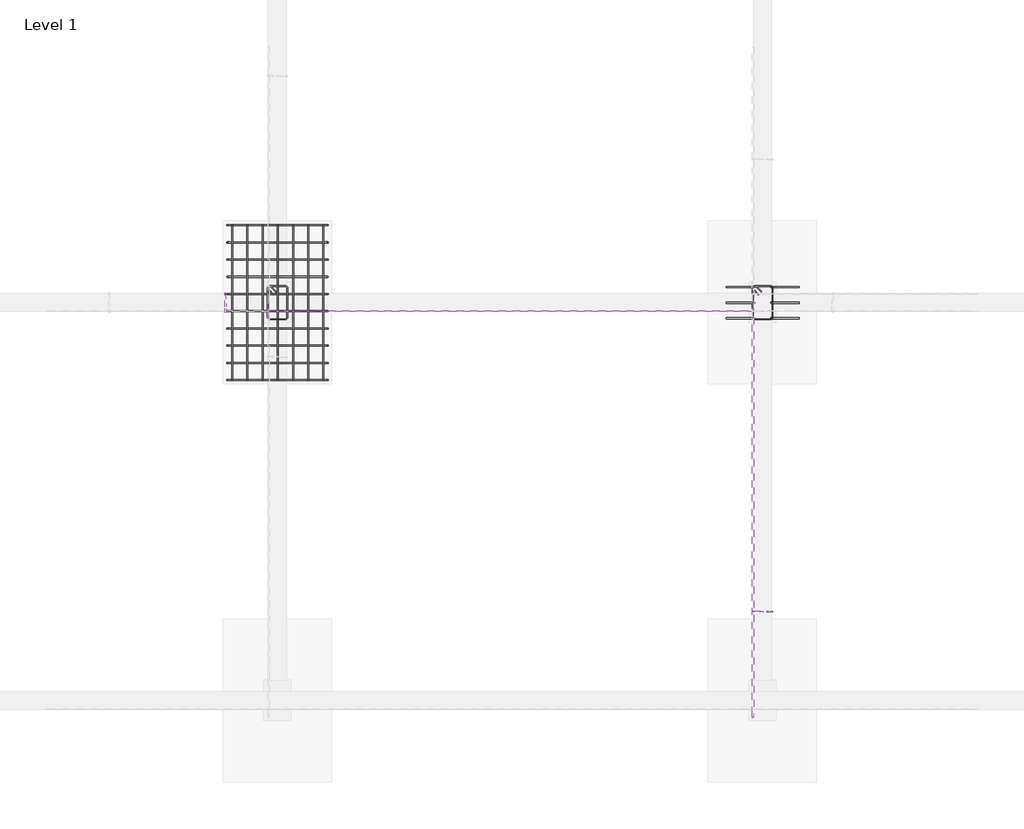
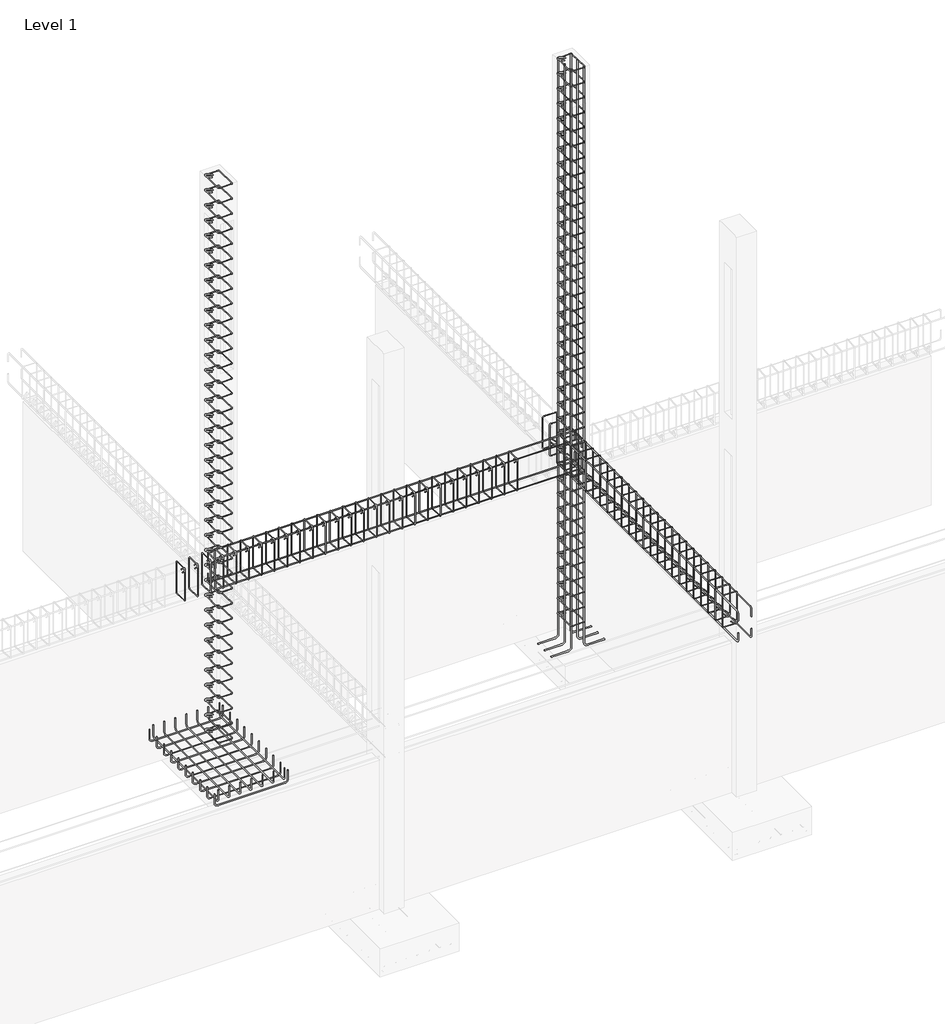
# One storey, part 5 of 8: 12 reinforcing bars.
"""IFC4 building model written with IfcOpenShell, lengths in millimetres."""

from ifc_helpers import new_model, si_unit, point, frame, origin, place, context, project, spatial, polyline, circle_curve, trimmed, segment, composite_curve, source, transform, mapped, element, save
from ifc_brep_helpers import swept_disk

model = new_model("IFC4")

# Units and contexts
model_context = context("Model", 3, world=origin())
ifc_project = project(units=[si_unit("LENGTHUNIT", "METRE", prefix="MILLI")], contexts=[model_context])

# Site, building, storey
site = spatial("IfcSite", under=ifc_project)
building = spatial("IfcBuilding", under=site)
storey = spatial("IfcBuildingStorey", under=building, Name="Level 1", Elevation=0.0)

# Reinforcing bars
placement = place(None, origin())
reinforcing_bar_shape = source(origin(), model_context, "Body", "SolidModel", [
    swept_disk(composite_curve([segment(polyline([(-8817.2482157, 7767.9070829, 9105.9), (-8817.2482157, 7767.9070829, -307.9115)]), True, "CONTINUOUS"), segment(trimmed(circle_curve(frame((-8771.1472157, 7767.9070829, -307.9115), z_axis=(0.0, -1.0, 0.0), x_axis=(-46.10099999999875, 0.0, 0.0)), 46.101), [point((-8817.2482157, 7767.9070829, -307.9115))], [point((-8771.1472157, 7767.9070829, -354.0125))], True, "CARTESIAN"), True, "CONTINUOUS"), segment(polyline([(-8771.1472157, 7767.9070829, -354.0125), (-8504.5742157, 7767.9070829, -354.0125)]), True, "CONTINUOUS")], self_intersect=False), 8.001),
])
element("IfcReinforcingBar", 1, at=placement, inside=storey, context=model_context, shape_type="MappedRepresentation", body=[
    mapped(reinforcing_bar_shape, transform((0.0, 0.0, 0.0), x_axis=(1.0, 0.0, 0.0), y_axis=(0.0, 1.0, 0.0), z_axis=(0.0, 0.0, 1.0))),
    mapped(reinforcing_bar_shape, transform((0.0, -174.625, 0.0), x_axis=(1.0, 0.0, 0.0), y_axis=(0.0, 1.0, 0.0), z_axis=(0.0, 0.0, 1.0))),
    mapped(reinforcing_bar_shape, transform((0.0, -349.25, 0.0), x_axis=(1.0, 0.0, 0.0), y_axis=(0.0, 1.0, 0.0), z_axis=(0.0, 0.0, 1.0))),
])
reinforcing_bar_2_shape = source(origin(), model_context, "Body", "SolidModel", [
    swept_disk(composite_curve([segment(polyline([(-9326.7722157, 7767.9070829, -354.0125), (-9060.1992157, 7767.9070829, -354.0125)]), True, "CONTINUOUS"), segment(trimmed(circle_curve(frame((-9060.1992157, 7767.9070829, -307.9115), z_axis=(0.0, -1.0, 0.0), x_axis=(0.0, 0.0, -46.101)), 46.101), [point((-9060.1992157, 7767.9070829, -354.0125))], [point((-9014.0982157, 7767.9070829, -307.9115))], True, "CARTESIAN"), True, "CONTINUOUS"), segment(polyline([(-9014.0982157, 7767.9070829, -307.9115), (-9014.0982157, 7767.9070829, 9105.9)]), True, "CONTINUOUS")], self_intersect=False), 8.001),
])
element("IfcReinforcingBar", 2, at=placement, inside=storey, context=model_context, shape_type="MappedRepresentation", body=[
    mapped(reinforcing_bar_2_shape, transform((0.0, 0.0, 0.0), x_axis=(1.0, 0.0, 0.0), y_axis=(0.0, 1.0, 0.0), z_axis=(0.0, 0.0, 1.0))),
    mapped(reinforcing_bar_2_shape, transform((0.0, -174.625, 0.0), x_axis=(1.0, 0.0, 0.0), y_axis=(0.0, 1.0, 0.0), z_axis=(0.0, 0.0, 1.0))),
    mapped(reinforcing_bar_2_shape, transform((0.0, -349.25, 0.0), x_axis=(1.0, 0.0, 0.0), y_axis=(0.0, 1.0, 0.0), z_axis=(0.0, 0.0, 1.0))),
])
reinforcing_bar_3_shape = source(origin(), model_context, "Body", "SolidModel", [
    swept_disk(composite_curve([segment(polyline([(-8929.9307551, 7716.2481494, 42.037), (-8986.7949521, 7773.1123465, 42.037)]), True, "CONTINUOUS"), segment(trimmed(circle_curve(frame((-9003.0492157, 7756.8580829, 42.037), z_axis=(0.0, 0.0, 1.0), x_axis=(16.25426360000165, 16.25426359999983, 0.0)), 22.987), [point((-8986.7949521, 7773.1123465, 42.037))], [point((-9026.0362157, 7756.8580829, 42.037))], True, "CARTESIAN"), True, "CONTINUOUS"), segment(polyline([(-9026.0362157, 7756.8580829, 42.037), (-9026.0362157, 7429.7060829, 42.037)]), True, "CONTINUOUS"), segment(trimmed(circle_curve(frame((-9003.0492157, 7429.7060829, 42.037), z_axis=(0.0, 0.0, 1.0), x_axis=(-22.98699999999917, 0.0, 0.0)), 22.987), [point((-9026.0362157, 7429.7060829, 42.037))], [point((-9003.0492157, 7406.7190829, 42.037))], True, "CARTESIAN"), True, "CONTINUOUS"), segment(polyline([(-9003.0492157, 7406.7190829, 42.037), (-8828.2972157, 7406.7190829, 42.037)]), True, "CONTINUOUS"), segment(trimmed(circle_curve(frame((-8828.2972157, 7429.7009662, 41.5520181), z_axis=(0.0, 0.02109809375347505, 0.9997774104469302), x_axis=(0.0, -22.981883299999936, 0.4849819000000011)), 22.987), [point((-8828.2972157, 7406.7190829, 42.037))], [point((-8805.3102157, 7429.7009662, 41.5520181))], True, "CARTESIAN"), True, "CONTINUOUS"), segment(polyline([(-8805.3102157, 7429.7009662, 41.5520181), (-8805.3102157, 7756.8631996, 34.6479819)]), True, "CONTINUOUS"), segment(trimmed(circle_curve(frame((-8828.2972157, 7756.8631996, 34.6479819), z_axis=(0.0, 0.02109809375347505, 0.9997774104469302), x_axis=(22.98700000000099, 0.0, 0.0)), 22.987), [point((-8805.3102157, 7756.8631996, 34.6479819))], [point((-8828.2972157, 7779.8450829, 34.163))], True, "CARTESIAN"), True, "CONTINUOUS"), segment(polyline([(-8828.2972157, 7779.8450829, 34.163), (-9003.0492157, 7779.8450829, 34.163)]), True, "CONTINUOUS"), segment(trimmed(circle_curve(frame((-9003.0492157, 7756.8580829, 34.163), z_axis=(0.0, 0.0, 1.0), x_axis=(0.0, 22.98700000000008, 0.0)), 22.987), [point((-9003.0492157, 7779.8450829, 34.163))], [point((-9019.3034793, 7740.6038193, 34.163))], True, "CARTESIAN"), True, "CONTINUOUS"), segment(polyline([(-9019.3034793, 7740.6038193, 34.163), (-8962.4392822, 7683.7396223, 34.163)]), True, "CONTINUOUS")], self_intersect=False), 3.937),
])
element("IfcReinforcingBar", 3, at=placement, inside=storey, context=model_context, shape_type="MappedRepresentation", body=[
    mapped(reinforcing_bar_3_shape, transform((0.0, 0.0, 0.0), x_axis=(1.0, 0.0, 0.0), y_axis=(0.0, 1.0, 0.0), z_axis=(0.0, 0.0, 1.0))),
    mapped(reinforcing_bar_3_shape, transform((0.0, 0.0, 244.8628649), x_axis=(1.0, 0.0, 0.0), y_axis=(0.0, 1.0, 0.0), z_axis=(0.0, 0.0, 1.0))),
    mapped(reinforcing_bar_3_shape, transform((0.0, 0.0, 489.7257297), x_axis=(1.0, 0.0, 0.0), y_axis=(0.0, 1.0, 0.0), z_axis=(0.0, 0.0, 1.0))),
    mapped(reinforcing_bar_3_shape, transform((0.0, 0.0, 734.5885946), x_axis=(1.0, 0.0, 0.0), y_axis=(0.0, 1.0, 0.0), z_axis=(0.0, 0.0, 1.0))),
    mapped(reinforcing_bar_3_shape, transform((0.0, 0.0, 979.4514595), x_axis=(1.0, 0.0, 0.0), y_axis=(0.0, 1.0, 0.0), z_axis=(0.0, 0.0, 1.0))),
    mapped(reinforcing_bar_3_shape, transform((0.0, 0.0, 1224.3143243), x_axis=(1.0, 0.0, 0.0), y_axis=(0.0, 1.0, 0.0), z_axis=(0.0, 0.0, 1.0))),
    mapped(reinforcing_bar_3_shape, transform((0.0, 0.0, 1469.1771892), x_axis=(1.0, 0.0, 0.0), y_axis=(0.0, 1.0, 0.0), z_axis=(0.0, 0.0, 1.0))),
    mapped(reinforcing_bar_3_shape, transform((0.0, 0.0, 1714.0400541), x_axis=(1.0, 0.0, 0.0), y_axis=(0.0, 1.0, 0.0), z_axis=(0.0, 0.0, 1.0))),
    mapped(reinforcing_bar_3_shape, transform((0.0, 0.0, 1958.9029189), x_axis=(1.0, 0.0, 0.0), y_axis=(0.0, 1.0, 0.0), z_axis=(0.0, 0.0, 1.0))),
    mapped(reinforcing_bar_3_shape, transform((0.0, 0.0, 2203.7657838), x_axis=(1.0, 0.0, 0.0), y_axis=(0.0, 1.0, 0.0), z_axis=(0.0, 0.0, 1.0))),
    mapped(reinforcing_bar_3_shape, transform((0.0, 0.0, 2448.6286486), x_axis=(1.0, 0.0, 0.0), y_axis=(0.0, 1.0, 0.0), z_axis=(0.0, 0.0, 1.0))),
    mapped(reinforcing_bar_3_shape, transform((0.0, 0.0, 2693.4915135), x_axis=(1.0, 0.0, 0.0), y_axis=(0.0, 1.0, 0.0), z_axis=(0.0, 0.0, 1.0))),
    mapped(reinforcing_bar_3_shape, transform((0.0, 0.0, 2938.3543784), x_axis=(1.0, 0.0, 0.0), y_axis=(0.0, 1.0, 0.0), z_axis=(0.0, 0.0, 1.0))),
    mapped(reinforcing_bar_3_shape, transform((0.0, 0.0, 3183.2172432), x_axis=(1.0, 0.0, 0.0), y_axis=(0.0, 1.0, 0.0), z_axis=(0.0, 0.0, 1.0))),
    mapped(reinforcing_bar_3_shape, transform((0.0, 0.0, 3428.0801081), x_axis=(1.0, 0.0, 0.0), y_axis=(0.0, 1.0, 0.0), z_axis=(0.0, 0.0, 1.0))),
    mapped(reinforcing_bar_3_shape, transform((0.0, 0.0, 3672.942973), x_axis=(1.0, 0.0, 0.0), y_axis=(0.0, 1.0, 0.0), z_axis=(0.0, 0.0, 1.0))),
    mapped(reinforcing_bar_3_shape, transform((0.0, 0.0, 3917.8058378), x_axis=(1.0, 0.0, 0.0), y_axis=(0.0, 1.0, 0.0), z_axis=(0.0, 0.0, 1.0))),
    mapped(reinforcing_bar_3_shape, transform((0.0, 0.0, 4162.6687027), x_axis=(1.0, 0.0, 0.0), y_axis=(0.0, 1.0, 0.0), z_axis=(0.0, 0.0, 1.0))),
    mapped(reinforcing_bar_3_shape, transform((0.0, 0.0, 4407.5315676), x_axis=(1.0, 0.0, 0.0), y_axis=(0.0, 1.0, 0.0), z_axis=(0.0, 0.0, 1.0))),
    mapped(reinforcing_bar_3_shape, transform((0.0, 0.0, 4652.3944324), x_axis=(1.0, 0.0, 0.0), y_axis=(0.0, 1.0, 0.0), z_axis=(0.0, 0.0, 1.0))),
    mapped(reinforcing_bar_3_shape, transform((0.0, 0.0, 4897.2572973), x_axis=(1.0, 0.0, 0.0), y_axis=(0.0, 1.0, 0.0), z_axis=(0.0, 0.0, 1.0))),
    mapped(reinforcing_bar_3_shape, transform((0.0, 0.0, 5142.1201622), x_axis=(1.0, 0.0, 0.0), y_axis=(0.0, 1.0, 0.0), z_axis=(0.0, 0.0, 1.0))),
    mapped(reinforcing_bar_3_shape, transform((0.0, 0.0, 5386.983027), x_axis=(1.0, 0.0, 0.0), y_axis=(0.0, 1.0, 0.0), z_axis=(0.0, 0.0, 1.0))),
    mapped(reinforcing_bar_3_shape, transform((0.0, 0.0, 5631.8458919), x_axis=(1.0, 0.0, 0.0), y_axis=(0.0, 1.0, 0.0), z_axis=(0.0, 0.0, 1.0))),
    mapped(reinforcing_bar_3_shape, transform((0.0, 0.0, 5876.7087568), x_axis=(1.0, 0.0, 0.0), y_axis=(0.0, 1.0, 0.0), z_axis=(0.0, 0.0, 1.0))),
    mapped(reinforcing_bar_3_shape, transform((0.0, 0.0, 6121.5716216), x_axis=(1.0, 0.0, 0.0), y_axis=(0.0, 1.0, 0.0), z_axis=(0.0, 0.0, 1.0))),
    mapped(reinforcing_bar_3_shape, transform((0.0, 0.0, 6366.4344865), x_axis=(1.0, 0.0, 0.0), y_axis=(0.0, 1.0, 0.0), z_axis=(0.0, 0.0, 1.0))),
    mapped(reinforcing_bar_3_shape, transform((0.0, 0.0, 6611.2973514), x_axis=(1.0, 0.0, 0.0), y_axis=(0.0, 1.0, 0.0), z_axis=(0.0, 0.0, 1.0))),
    mapped(reinforcing_bar_3_shape, transform((0.0, 0.0, 6856.1602162), x_axis=(1.0, 0.0, 0.0), y_axis=(0.0, 1.0, 0.0), z_axis=(0.0, 0.0, 1.0))),
    mapped(reinforcing_bar_3_shape, transform((0.0, 0.0, 7101.0230811), x_axis=(1.0, 0.0, 0.0), y_axis=(0.0, 1.0, 0.0), z_axis=(0.0, 0.0, 1.0))),
    mapped(reinforcing_bar_3_shape, transform((0.0, 0.0, 7345.8859459), x_axis=(1.0, 0.0, 0.0), y_axis=(0.0, 1.0, 0.0), z_axis=(0.0, 0.0, 1.0))),
    mapped(reinforcing_bar_3_shape, transform((0.0, 0.0, 7590.7488108), x_axis=(1.0, 0.0, 0.0), y_axis=(0.0, 1.0, 0.0), z_axis=(0.0, 0.0, 1.0))),
    mapped(reinforcing_bar_3_shape, transform((0.0, 0.0, 7835.6116757), x_axis=(1.0, 0.0, 0.0), y_axis=(0.0, 1.0, 0.0), z_axis=(0.0, 0.0, 1.0))),
    mapped(reinforcing_bar_3_shape, transform((0.0, 0.0, 8080.4745405), x_axis=(1.0, 0.0, 0.0), y_axis=(0.0, 1.0, 0.0), z_axis=(0.0, 0.0, 1.0))),
    mapped(reinforcing_bar_3_shape, transform((0.0, 0.0, 8325.3374054), x_axis=(1.0, 0.0, 0.0), y_axis=(0.0, 1.0, 0.0), z_axis=(0.0, 0.0, 1.0))),
    mapped(reinforcing_bar_3_shape, transform((0.0, 0.0, 8570.2002703), x_axis=(1.0, 0.0, 0.0), y_axis=(0.0, 1.0, 0.0), z_axis=(0.0, 0.0, 1.0))),
    mapped(reinforcing_bar_3_shape, transform((0.0, 0.0, 8815.0631351), x_axis=(1.0, 0.0, 0.0), y_axis=(0.0, 1.0, 0.0), z_axis=(0.0, 0.0, 1.0))),
    mapped(reinforcing_bar_3_shape, transform((0.0, 0.0, 9059.926), x_axis=(1.0, 0.0, 0.0), y_axis=(0.0, 1.0, 0.0), z_axis=(0.0, 0.0, 1.0))),
])
reinforcing_bar_4_shape = source(origin(), model_context, "Body", "SolidModel", [
    swept_disk(composite_curve([segment(polyline([(-14375.7176938, 7716.2481494, 42.037), (-14432.5818909, 7773.1123465, 42.037)]), True, "CONTINUOUS"), segment(trimmed(circle_curve(frame((-14448.8361545, 7756.8580829, 42.037), z_axis=(0.0, 0.0, 1.0), x_axis=(16.25426359999983, 16.25426359999983, 0.0)), 22.987), [point((-14432.5818909, 7773.1123465, 42.037))], [point((-14471.8231545, 7756.8580829, 42.037))], True, "CARTESIAN"), True, "CONTINUOUS"), segment(polyline([(-14471.8231545, 7756.8580829, 42.037), (-14471.8231545, 7429.7060829, 42.037)]), True, "CONTINUOUS"), segment(trimmed(circle_curve(frame((-14448.8361545, 7429.7060829, 42.037), z_axis=(0.0, 0.0, 1.0), x_axis=(-22.98699999999917, 0.0, 0.0)), 22.987), [point((-14471.8231545, 7429.7060829, 42.037))], [point((-14448.8361545, 7406.7190829, 42.037))], True, "CARTESIAN"), True, "CONTINUOUS"), segment(polyline([(-14448.8361545, 7406.7190829, 42.037), (-14274.0841545, 7406.7190829, 42.037)]), True, "CONTINUOUS"), segment(trimmed(circle_curve(frame((-14274.0841545, 7429.7009662, 41.5520181), z_axis=(0.0, 0.02109809375347505, 0.9997774104469302), x_axis=(0.0, -22.981883299999936, 0.4849819000000011)), 22.987), [point((-14274.0841545, 7406.7190829, 42.037))], [point((-14251.0971545, 7429.7009662, 41.5520181))], True, "CARTESIAN"), True, "CONTINUOUS"), segment(polyline([(-14251.0971545, 7429.7009662, 41.5520181), (-14251.0971545, 7756.8631996, 34.6479819)]), True, "CONTINUOUS"), segment(trimmed(circle_curve(frame((-14274.0841545, 7756.8631996, 34.6479819), z_axis=(0.0, 0.02109809375347505, 0.9997774104469302), x_axis=(22.98700000000099, 0.0, 0.0)), 22.987), [point((-14251.0971545, 7756.8631996, 34.6479819))], [point((-14274.0841545, 7779.8450829, 34.163))], True, "CARTESIAN"), True, "CONTINUOUS"), segment(polyline([(-14274.0841545, 7779.8450829, 34.163), (-14448.8361545, 7779.8450829, 34.163)]), True, "CONTINUOUS"), segment(trimmed(circle_curve(frame((-14448.8361545, 7756.8580829, 34.163), z_axis=(0.0, 0.0, 1.0), x_axis=(0.0, 22.98700000000008, 0.0)), 22.987), [point((-14448.8361545, 7779.8450829, 34.163))], [point((-14465.0904181, 7740.6038193, 34.163))], True, "CARTESIAN"), True, "CONTINUOUS"), segment(polyline([(-14465.0904181, 7740.6038193, 34.163), (-14408.226221, 7683.7396223, 34.163)]), True, "CONTINUOUS")], self_intersect=False), 3.937),
])
element("IfcReinforcingBar", 4, at=placement, inside=storey, context=model_context, shape_type="MappedRepresentation", body=[
    mapped(reinforcing_bar_4_shape, transform((0.0, 0.0, 0.0), x_axis=(1.0, 0.0, 0.0), y_axis=(0.0, 1.0, 0.0), z_axis=(0.0, 0.0, 1.0))),
    mapped(reinforcing_bar_4_shape, transform((0.0, 0.0, 244.8628649), x_axis=(1.0, 0.0, 0.0), y_axis=(0.0, 1.0, 0.0), z_axis=(0.0, 0.0, 1.0))),
    mapped(reinforcing_bar_4_shape, transform((0.0, 0.0, 489.7257297), x_axis=(1.0, 0.0, 0.0), y_axis=(0.0, 1.0, 0.0), z_axis=(0.0, 0.0, 1.0))),
    mapped(reinforcing_bar_4_shape, transform((0.0, 0.0, 734.5885946), x_axis=(1.0, 0.0, 0.0), y_axis=(0.0, 1.0, 0.0), z_axis=(0.0, 0.0, 1.0))),
    mapped(reinforcing_bar_4_shape, transform((0.0, 0.0, 979.4514595), x_axis=(1.0, 0.0, 0.0), y_axis=(0.0, 1.0, 0.0), z_axis=(0.0, 0.0, 1.0))),
    mapped(reinforcing_bar_4_shape, transform((0.0, 0.0, 1224.3143243), x_axis=(1.0, 0.0, 0.0), y_axis=(0.0, 1.0, 0.0), z_axis=(0.0, 0.0, 1.0))),
    mapped(reinforcing_bar_4_shape, transform((0.0, 0.0, 1469.1771892), x_axis=(1.0, 0.0, 0.0), y_axis=(0.0, 1.0, 0.0), z_axis=(0.0, 0.0, 1.0))),
    mapped(reinforcing_bar_4_shape, transform((0.0, 0.0, 1714.0400541), x_axis=(1.0, 0.0, 0.0), y_axis=(0.0, 1.0, 0.0), z_axis=(0.0, 0.0, 1.0))),
    mapped(reinforcing_bar_4_shape, transform((0.0, 0.0, 1958.9029189), x_axis=(1.0, 0.0, 0.0), y_axis=(0.0, 1.0, 0.0), z_axis=(0.0, 0.0, 1.0))),
    mapped(reinforcing_bar_4_shape, transform((0.0, 0.0, 2203.7657838), x_axis=(1.0, 0.0, 0.0), y_axis=(0.0, 1.0, 0.0), z_axis=(0.0, 0.0, 1.0))),
    mapped(reinforcing_bar_4_shape, transform((0.0, 0.0, 2448.6286486), x_axis=(1.0, 0.0, 0.0), y_axis=(0.0, 1.0, 0.0), z_axis=(0.0, 0.0, 1.0))),
    mapped(reinforcing_bar_4_shape, transform((0.0, 0.0, 2693.4915135), x_axis=(1.0, 0.0, 0.0), y_axis=(0.0, 1.0, 0.0), z_axis=(0.0, 0.0, 1.0))),
    mapped(reinforcing_bar_4_shape, transform((0.0, 0.0, 2938.3543784), x_axis=(1.0, 0.0, 0.0), y_axis=(0.0, 1.0, 0.0), z_axis=(0.0, 0.0, 1.0))),
    mapped(reinforcing_bar_4_shape, transform((0.0, 0.0, 3183.2172432), x_axis=(1.0, 0.0, 0.0), y_axis=(0.0, 1.0, 0.0), z_axis=(0.0, 0.0, 1.0))),
    mapped(reinforcing_bar_4_shape, transform((0.0, 0.0, 3428.0801081), x_axis=(1.0, 0.0, 0.0), y_axis=(0.0, 1.0, 0.0), z_axis=(0.0, 0.0, 1.0))),
    mapped(reinforcing_bar_4_shape, transform((0.0, 0.0, 3672.942973), x_axis=(1.0, 0.0, 0.0), y_axis=(0.0, 1.0, 0.0), z_axis=(0.0, 0.0, 1.0))),
    mapped(reinforcing_bar_4_shape, transform((0.0, 0.0, 3917.8058378), x_axis=(1.0, 0.0, 0.0), y_axis=(0.0, 1.0, 0.0), z_axis=(0.0, 0.0, 1.0))),
    mapped(reinforcing_bar_4_shape, transform((0.0, 0.0, 4162.6687027), x_axis=(1.0, 0.0, 0.0), y_axis=(0.0, 1.0, 0.0), z_axis=(0.0, 0.0, 1.0))),
    mapped(reinforcing_bar_4_shape, transform((0.0, 0.0, 4407.5315676), x_axis=(1.0, 0.0, 0.0), y_axis=(0.0, 1.0, 0.0), z_axis=(0.0, 0.0, 1.0))),
    mapped(reinforcing_bar_4_shape, transform((0.0, 0.0, 4652.3944324), x_axis=(1.0, 0.0, 0.0), y_axis=(0.0, 1.0, 0.0), z_axis=(0.0, 0.0, 1.0))),
    mapped(reinforcing_bar_4_shape, transform((0.0, 0.0, 4897.2572973), x_axis=(1.0, 0.0, 0.0), y_axis=(0.0, 1.0, 0.0), z_axis=(0.0, 0.0, 1.0))),
    mapped(reinforcing_bar_4_shape, transform((0.0, 0.0, 5142.1201622), x_axis=(1.0, 0.0, 0.0), y_axis=(0.0, 1.0, 0.0), z_axis=(0.0, 0.0, 1.0))),
    mapped(reinforcing_bar_4_shape, transform((0.0, 0.0, 5386.983027), x_axis=(1.0, 0.0, 0.0), y_axis=(0.0, 1.0, 0.0), z_axis=(0.0, 0.0, 1.0))),
    mapped(reinforcing_bar_4_shape, transform((0.0, 0.0, 5631.8458919), x_axis=(1.0, 0.0, 0.0), y_axis=(0.0, 1.0, 0.0), z_axis=(0.0, 0.0, 1.0))),
    mapped(reinforcing_bar_4_shape, transform((0.0, 0.0, 5876.7087568), x_axis=(1.0, 0.0, 0.0), y_axis=(0.0, 1.0, 0.0), z_axis=(0.0, 0.0, 1.0))),
    mapped(reinforcing_bar_4_shape, transform((0.0, 0.0, 6121.5716216), x_axis=(1.0, 0.0, 0.0), y_axis=(0.0, 1.0, 0.0), z_axis=(0.0, 0.0, 1.0))),
    mapped(reinforcing_bar_4_shape, transform((0.0, 0.0, 6366.4344865), x_axis=(1.0, 0.0, 0.0), y_axis=(0.0, 1.0, 0.0), z_axis=(0.0, 0.0, 1.0))),
    mapped(reinforcing_bar_4_shape, transform((0.0, 0.0, 6611.2973514), x_axis=(1.0, 0.0, 0.0), y_axis=(0.0, 1.0, 0.0), z_axis=(0.0, 0.0, 1.0))),
    mapped(reinforcing_bar_4_shape, transform((0.0, 0.0, 6856.1602162), x_axis=(1.0, 0.0, 0.0), y_axis=(0.0, 1.0, 0.0), z_axis=(0.0, 0.0, 1.0))),
    mapped(reinforcing_bar_4_shape, transform((0.0, 0.0, 7101.0230811), x_axis=(1.0, 0.0, 0.0), y_axis=(0.0, 1.0, 0.0), z_axis=(0.0, 0.0, 1.0))),
    mapped(reinforcing_bar_4_shape, transform((0.0, 0.0, 7345.8859459), x_axis=(1.0, 0.0, 0.0), y_axis=(0.0, 1.0, 0.0), z_axis=(0.0, 0.0, 1.0))),
    mapped(reinforcing_bar_4_shape, transform((0.0, 0.0, 7590.7488108), x_axis=(1.0, 0.0, 0.0), y_axis=(0.0, 1.0, 0.0), z_axis=(0.0, 0.0, 1.0))),
    mapped(reinforcing_bar_4_shape, transform((0.0, 0.0, 7835.6116757), x_axis=(1.0, 0.0, 0.0), y_axis=(0.0, 1.0, 0.0), z_axis=(0.0, 0.0, 1.0))),
    mapped(reinforcing_bar_4_shape, transform((0.0, 0.0, 8080.4745405), x_axis=(1.0, 0.0, 0.0), y_axis=(0.0, 1.0, 0.0), z_axis=(0.0, 0.0, 1.0))),
    mapped(reinforcing_bar_4_shape, transform((0.0, 0.0, 8325.3374054), x_axis=(1.0, 0.0, 0.0), y_axis=(0.0, 1.0, 0.0), z_axis=(0.0, 0.0, 1.0))),
    mapped(reinforcing_bar_4_shape, transform((0.0, 0.0, 8570.2002703), x_axis=(1.0, 0.0, 0.0), y_axis=(0.0, 1.0, 0.0), z_axis=(0.0, 0.0, 1.0))),
    mapped(reinforcing_bar_4_shape, transform((0.0, 0.0, 8815.0631351), x_axis=(1.0, 0.0, 0.0), y_axis=(0.0, 1.0, 0.0), z_axis=(0.0, 0.0, 1.0))),
    mapped(reinforcing_bar_4_shape, transform((0.0, 0.0, 9059.926), x_axis=(1.0, 0.0, 0.0), y_axis=(0.0, 1.0, 0.0), z_axis=(0.0, 0.0, 1.0))),
])
reinforcing_bar_5_shape = source(origin(), model_context, "Body", "SolidModel", [
    swept_disk(composite_curve([segment(polyline([(-13795.9291545, 8463.6130829, -216.662), (-13795.9291545, 8463.6130829, -369.062)]), True, "CONTINUOUS"), segment(trimmed(circle_curve(frame((-13839.9981545, 8463.6130829, -369.062), z_axis=(0.0, 1.0, 0.0), x_axis=(44.068999999999505, 0.0, 0.0)), 44.069), [point((-13795.9291545, 8463.6130829, -369.062))], [point((-13839.9981545, 8463.6130829, -413.131))], True, "CARTESIAN"), True, "CONTINUOUS"), segment(polyline([(-13839.9981545, 8463.6130829, -413.131), (-14882.9221545, 8463.6130829, -413.131)]), True, "CONTINUOUS"), segment(trimmed(circle_curve(frame((-14882.9221545, 8463.6130829, -369.062), z_axis=(0.0, 1.0, 0.0), x_axis=(0.0, 0.0, -44.06899999999996)), 44.069), [point((-14882.9221545, 8463.6130829, -413.131))], [point((-14926.9911545, 8463.6130829, -369.062))], True, "CARTESIAN"), True, "CONTINUOUS"), segment(polyline([(-14926.9911545, 8463.6130829, -369.062), (-14926.9911545, 8463.6130829, -216.662)]), True, "CONTINUOUS")], self_intersect=False), 5.969),
])
element("IfcReinforcingBar", 5, at=placement, inside=storey, context=model_context, shape_type="MappedRepresentation", body=[
    mapped(reinforcing_bar_5_shape, transform((0.0, 0.0, 0.0), x_axis=(1.0, 0.0, 0.0), y_axis=(0.0, 1.0, 0.0), z_axis=(0.0, 0.0, 1.0))),
    mapped(reinforcing_bar_5_shape, transform((0.0, -193.4068889, 0.0), x_axis=(1.0, 0.0, 0.0), y_axis=(0.0, 1.0, 0.0), z_axis=(0.0, 0.0, 1.0))),
    mapped(reinforcing_bar_5_shape, transform((0.0, -386.8137778, 0.0), x_axis=(1.0, 0.0, 0.0), y_axis=(0.0, 1.0, 0.0), z_axis=(0.0, 0.0, 1.0))),
    mapped(reinforcing_bar_5_shape, transform((0.0, -580.2206667, 0.0), x_axis=(1.0, 0.0, 0.0), y_axis=(0.0, 1.0, 0.0), z_axis=(0.0, 0.0, 1.0))),
    mapped(reinforcing_bar_5_shape, transform((0.0, -773.6275556, 0.0), x_axis=(1.0, 0.0, 0.0), y_axis=(0.0, 1.0, 0.0), z_axis=(0.0, 0.0, 1.0))),
    mapped(reinforcing_bar_5_shape, transform((0.0, -967.0344444, 0.0), x_axis=(1.0, 0.0, 0.0), y_axis=(0.0, 1.0, 0.0), z_axis=(0.0, 0.0, 1.0))),
    mapped(reinforcing_bar_5_shape, transform((0.0, -1160.4413333, 0.0), x_axis=(1.0, 0.0, 0.0), y_axis=(0.0, 1.0, 0.0), z_axis=(0.0, 0.0, 1.0))),
    mapped(reinforcing_bar_5_shape, transform((0.0, -1353.8482222, 0.0), x_axis=(1.0, 0.0, 0.0), y_axis=(0.0, 1.0, 0.0), z_axis=(0.0, 0.0, 1.0))),
    mapped(reinforcing_bar_5_shape, transform((0.0, -1547.2551111, 0.0), x_axis=(1.0, 0.0, 0.0), y_axis=(0.0, 1.0, 0.0), z_axis=(0.0, 0.0, 1.0))),
    mapped(reinforcing_bar_5_shape, transform((0.0, -1740.662, 0.0), x_axis=(1.0, 0.0, 0.0), y_axis=(0.0, 1.0, 0.0), z_axis=(0.0, 0.0, 1.0))),
])
reinforcing_bar_6_shape = source(origin(), model_context, "Body", "SolidModel", [
    swept_disk(composite_curve([segment(polyline([(-14869.4601545, 8463.6130829, -165.481), (-14869.4601545, 8463.6130829, -317.881)]), True, "CONTINUOUS"), segment(trimmed(circle_curve(frame((-14869.4601545, 8419.5440829, -317.881), z_axis=(-1.0, 0.0, 0.0), x_axis=(0.0, 44.068999999999505, 0.0)), 44.069), [point((-14869.4601545, 8463.6130829, -317.881))], [point((-14869.4601545, 8419.5440829, -361.95))], True, "CARTESIAN"), True, "CONTINUOUS"), segment(polyline([(-14869.4601545, 8419.5440829, -361.95), (-14869.4601545, 6767.0200829, -361.95)]), True, "CONTINUOUS"), segment(trimmed(circle_curve(frame((-14869.4601545, 6767.0200829, -317.881), z_axis=(-1.0, 0.0, 0.0), x_axis=(0.0, 0.0, -44.06900000000002)), 44.069), [point((-14869.4601545, 6767.0200829, -361.95))], [point((-14869.4601545, 6722.9510829, -317.881))], True, "CARTESIAN"), True, "CONTINUOUS"), segment(polyline([(-14869.4601545, 6722.9510829, -317.881), (-14869.4601545, 6722.9510829, -165.481)]), True, "CONTINUOUS")], self_intersect=False), 5.969),
])
element("IfcReinforcingBar", 6, at=placement, inside=storey, context=model_context, shape_type="MappedRepresentation", body=[
    mapped(reinforcing_bar_6_shape, transform((0.0, 0.0, 0.0), x_axis=(1.0, 0.0, 0.0), y_axis=(0.0, 1.0, 0.0), z_axis=(0.0, 0.0, 1.0))),
    mapped(reinforcing_bar_6_shape, transform((170.5954914, 0.0, 0.0), x_axis=(1.0, 0.0, 0.0), y_axis=(0.0, 1.0, 0.0), z_axis=(0.0, 0.0, 1.0))),
    mapped(reinforcing_bar_6_shape, transform((341.1909829, 0.0, 0.0), x_axis=(1.0, 0.0, 0.0), y_axis=(0.0, 1.0, 0.0), z_axis=(0.0, 0.0, 1.0))),
    mapped(reinforcing_bar_6_shape, transform((511.7864743, 0.0, 0.0), x_axis=(1.0, 0.0, 0.0), y_axis=(0.0, 1.0, 0.0), z_axis=(0.0, 0.0, 1.0))),
    mapped(reinforcing_bar_6_shape, transform((682.3819658, 0.0, 0.0), x_axis=(1.0, 0.0, 0.0), y_axis=(0.0, 1.0, 0.0), z_axis=(0.0, 0.0, 1.0))),
    mapped(reinforcing_bar_6_shape, transform((852.9774572, 0.0, 0.0), x_axis=(1.0, 0.0, 0.0), y_axis=(0.0, 1.0, 0.0), z_axis=(0.0, 0.0, 1.0))),
    mapped(reinforcing_bar_6_shape, transform((1023.5729487, 0.0, 0.0), x_axis=(1.0, 0.0, 0.0), y_axis=(0.0, 1.0, 0.0), z_axis=(0.0, 0.0, 1.0))),
])
reinforcing_bar_7_shape = source(origin(), model_context, "Body", "SolidModel", [
    swept_disk(composite_curve([segment(polyline([(-14469.7911545, 7496.6564191, 2643.0183362), (-14469.7911545, 7496.6564191, 2528.7183362)]), True, "CONTINUOUS"), segment(trimmed(circle_curve(frame((-14435.2471545, 7496.6564191, 2528.7183362), z_axis=(0.0, -1.0, 0.0), x_axis=(-34.54399999999987, 0.0, 0.0)), 34.544), [point((-14469.7911545, 7496.6564191, 2528.7183362))], [point((-14435.2471545, 7496.6564191, 2494.1743362))], True, "CARTESIAN"), True, "CONTINUOUS"), segment(polyline([(-14435.2471545, 7496.6564191, 2494.1743362), (-8841.8862157, 7496.6564191, 2494.1743362)]), True, "CONTINUOUS"), segment(trimmed(circle_curve(frame((-8841.8862157, 7496.6564191, 2528.7183362), z_axis=(0.0, -1.0, 0.0), x_axis=(0.0, 0.0, -34.54399999999987)), 34.544), [point((-8841.8862157, 7496.6564191, 2494.1743362))], [point((-8807.3422157, 7496.6564191, 2528.7183362))], True, "CARTESIAN"), True, "CONTINUOUS"), segment(polyline([(-8807.3422157, 7496.6564191, 2528.7183362), (-8807.3422157, 7496.6564191, 2643.0183362)]), True, "CONTINUOUS")], self_intersect=False), 5.969),
])
element("IfcReinforcingBar", 7, at=placement, inside=storey, context=model_context, shape_type="MappedRepresentation", body=[
    mapped(reinforcing_bar_7_shape, transform((0.0, 0.0, 0.0), x_axis=(1.0, 0.0, 0.0), y_axis=(0.0, 1.0, 0.0), z_axis=(0.0, 0.0, 1.0))),
    mapped(reinforcing_bar_7_shape, transform((0.0, 193.2513276, 0.0), x_axis=(1.0, 0.0, 0.0), y_axis=(0.0, 1.0, 0.0), z_axis=(0.0, 0.0, 1.0))),
])
reinforcing_bar_8_shape = source(origin(), model_context, "Body", "SolidModel", [
    swept_disk(composite_curve([segment(polyline([(-8807.3422157, 7496.6564191, 2843.3816638), (-8807.3422157, 7496.6564191, 2957.6816638)]), True, "CONTINUOUS"), segment(trimmed(circle_curve(frame((-8841.8862157, 7496.6564191, 2957.6816638), z_axis=(0.0, -1.0, 0.0), x_axis=(34.54399999999987, 0.0, 0.0)), 34.544), [point((-8807.3422157, 7496.6564191, 2957.6816638))], [point((-8841.8862157, 7496.6564191, 2992.2256638))], True, "CARTESIAN"), True, "CONTINUOUS"), segment(polyline([(-8841.8862157, 7496.6564191, 2992.2256638), (-14435.2471545, 7496.6564191, 2992.2256638)]), True, "CONTINUOUS"), segment(trimmed(circle_curve(frame((-14435.2471545, 7496.6564191, 2957.6816638), z_axis=(0.0, -1.0, 0.0), x_axis=(0.0, 0.0, 34.54399999999987)), 34.544), [point((-14435.2471545, 7496.6564191, 2992.2256638))], [point((-14469.7911545, 7496.6564191, 2957.6816638))], True, "CARTESIAN"), True, "CONTINUOUS"), segment(polyline([(-14469.7911545, 7496.6564191, 2957.6816638), (-14469.7911545, 7496.6564191, 2843.3816638)]), True, "CONTINUOUS")], self_intersect=False), 5.969),
])
element("IfcReinforcingBar", 8, at=placement, inside=storey, context=model_context, shape_type="MappedRepresentation", body=[
    mapped(reinforcing_bar_8_shape, transform((0.0, 0.0, 0.0), x_axis=(1.0, 0.0, 0.0), y_axis=(0.0, 1.0, 0.0), z_axis=(0.0, 0.0, 1.0))),
    mapped(reinforcing_bar_8_shape, transform((0.0, 193.2513276, 0.0), x_axis=(1.0, 0.0, 0.0), y_axis=(0.0, 1.0, 0.0), z_axis=(0.0, 0.0, 1.0))),
])
reinforcing_bar_9_shape = source(origin(), model_context, "Body", "SolidModel", [
    swept_disk(composite_curve([segment(polyline([(-9816.8708704, 7546.5160164, 2909.8575394), (-9816.8708704, 7489.6518193, 2966.7217364)]), True, "CONTINUOUS"), segment(trimmed(circle_curve(frame((-9816.8708704, 7505.9060829, 2982.976), z_axis=(-1.0, 0.0, 0.0), x_axis=(0.0, -16.25426359999983, -16.254263600000286)), 22.987), [point((-9816.8708704, 7489.6518193, 2966.7217364))], [point((-9816.8708704, 7505.9060829, 3005.963))], True, "CARTESIAN"), True, "CONTINUOUS"), segment(polyline([(-9816.8708704, 7505.9060829, 3005.963), (-9816.8708704, 7680.6580829, 3005.963)]), True, "CONTINUOUS"), segment(trimmed(circle_curve(frame((-9816.8708704, 7680.6580829, 2982.976), z_axis=(-1.0, 0.0, 0.0), x_axis=(0.0, 0.0, 22.98700000000008)), 22.987), [point((-9816.8708704, 7680.6580829, 3005.963))], [point((-9816.8708704, 7703.6450829, 2982.976))], True, "CARTESIAN"), True, "CONTINUOUS"), segment(polyline([(-9816.8708704, 7703.6450829, 2982.976), (-9816.8708704, 7703.6450829, 2503.424)]), True, "CONTINUOUS"), segment(trimmed(circle_curve(frame((-9816.0513721, 7680.6726953, 2503.424), z_axis=(-0.9993643184948482, -0.035650510786349336, 0.0), x_axis=(-0.8194982999993954, 22.97238759999982, 0.0)), 22.987), [point((-9816.8708704, 7703.6450829, 2503.424))], [point((-9816.0513721, 7680.6726953, 2480.437))], True, "CARTESIAN"), True, "CONTINUOUS"), segment(polyline([(-9816.0513721, 7680.6726953, 2480.437), (-9809.8163687, 7505.8914705, 2480.437)]), True, "CONTINUOUS"), segment(trimmed(circle_curve(frame((-9809.8163687, 7505.8914705, 2503.424), z_axis=(-0.9993643184948482, -0.035650510786349336, 0.0), x_axis=(0.0, 0.0, -22.98700000000008)), 22.987), [point((-9809.8163687, 7505.8914705, 2480.437))], [point((-9808.9968704, 7482.9190829, 2503.424))], True, "CARTESIAN"), True, "CONTINUOUS"), segment(polyline([(-9808.9968704, 7482.9190829, 2503.424), (-9808.9968704, 7482.9190829, 2982.976)]), True, "CONTINUOUS"), segment(trimmed(circle_curve(frame((-9808.9968704, 7505.9060829, 2982.976), z_axis=(-1.0, 0.0, 0.0), x_axis=(0.0, -22.98700000000008, 0.0)), 22.987), [point((-9808.9968704, 7482.9190829, 2982.976))], [point((-9808.9968704, 7522.1603465, 2999.2302636))], True, "CARTESIAN"), True, "CONTINUOUS"), segment(polyline([(-9808.9968704, 7522.1603465, 2999.2302636), (-9808.9968704, 7579.0245435, 2942.3660665)]), True, "CONTINUOUS")], self_intersect=False), 3.937),
])
element("IfcReinforcingBar", 9, at=placement, inside=storey, context=model_context, shape_type="MappedRepresentation", body=[
    mapped(reinforcing_bar_9_shape, transform((0.0, 0.0, 0.0), x_axis=(1.0, 0.0, 0.0), y_axis=(0.0, 1.0, 0.0), z_axis=(0.0, 0.0, 1.0))),
    mapped(reinforcing_bar_9_shape, transform((-197.4274207, 0.0, 0.0), x_axis=(1.0, 0.0, 0.0), y_axis=(0.0, 1.0, 0.0), z_axis=(0.0, 0.0, 1.0))),
    mapped(reinforcing_bar_9_shape, transform((-394.8548414, 0.0, 0.0), x_axis=(1.0, 0.0, 0.0), y_axis=(0.0, 1.0, 0.0), z_axis=(0.0, 0.0, 1.0))),
    mapped(reinforcing_bar_9_shape, transform((-592.2822622, 0.0, 0.0), x_axis=(1.0, 0.0, 0.0), y_axis=(0.0, 1.0, 0.0), z_axis=(0.0, 0.0, 1.0))),
    mapped(reinforcing_bar_9_shape, transform((-789.7096829, 0.0, 0.0), x_axis=(1.0, 0.0, 0.0), y_axis=(0.0, 1.0, 0.0), z_axis=(0.0, 0.0, 1.0))),
    mapped(reinforcing_bar_9_shape, transform((-987.1371036, 0.0, 0.0), x_axis=(1.0, 0.0, 0.0), y_axis=(0.0, 1.0, 0.0), z_axis=(0.0, 0.0, 1.0))),
    mapped(reinforcing_bar_9_shape, transform((-1184.5645243, 0.0, 0.0), x_axis=(1.0, 0.0, 0.0), y_axis=(0.0, 1.0, 0.0), z_axis=(0.0, 0.0, 1.0))),
    mapped(reinforcing_bar_9_shape, transform((-1381.991945, 0.0, 0.0), x_axis=(1.0, 0.0, 0.0), y_axis=(0.0, 1.0, 0.0), z_axis=(0.0, 0.0, 1.0))),
    mapped(reinforcing_bar_9_shape, transform((-1579.4193658, 0.0, 0.0), x_axis=(1.0, 0.0, 0.0), y_axis=(0.0, 1.0, 0.0), z_axis=(0.0, 0.0, 1.0))),
    mapped(reinforcing_bar_9_shape, transform((-1776.8467865, 0.0, 0.0), x_axis=(1.0, 0.0, 0.0), y_axis=(0.0, 1.0, 0.0), z_axis=(0.0, 0.0, 1.0))),
    mapped(reinforcing_bar_9_shape, transform((-1974.2742072, 0.0, 0.0), x_axis=(1.0, 0.0, 0.0), y_axis=(0.0, 1.0, 0.0), z_axis=(0.0, 0.0, 1.0))),
    mapped(reinforcing_bar_9_shape, transform((-2171.7016279, 0.0, 0.0), x_axis=(1.0, 0.0, 0.0), y_axis=(0.0, 1.0, 0.0), z_axis=(0.0, 0.0, 1.0))),
    mapped(reinforcing_bar_9_shape, transform((-2369.1290487, 0.0, 0.0), x_axis=(1.0, 0.0, 0.0), y_axis=(0.0, 1.0, 0.0), z_axis=(0.0, 0.0, 1.0))),
    mapped(reinforcing_bar_9_shape, transform((-2566.5564694, 0.0, 0.0), x_axis=(1.0, 0.0, 0.0), y_axis=(0.0, 1.0, 0.0), z_axis=(0.0, 0.0, 1.0))),
    mapped(reinforcing_bar_9_shape, transform((-2763.9838901, 0.0, 0.0), x_axis=(1.0, 0.0, 0.0), y_axis=(0.0, 1.0, 0.0), z_axis=(0.0, 0.0, 1.0))),
    mapped(reinforcing_bar_9_shape, transform((-2961.4113108, 0.0, 0.0), x_axis=(1.0, 0.0, 0.0), y_axis=(0.0, 1.0, 0.0), z_axis=(0.0, 0.0, 1.0))),
    mapped(reinforcing_bar_9_shape, transform((-3158.8387315, 0.0, 0.0), x_axis=(1.0, 0.0, 0.0), y_axis=(0.0, 1.0, 0.0), z_axis=(0.0, 0.0, 1.0))),
    mapped(reinforcing_bar_9_shape, transform((-3356.2661523, 0.0, 0.0), x_axis=(1.0, 0.0, 0.0), y_axis=(0.0, 1.0, 0.0), z_axis=(0.0, 0.0, 1.0))),
    mapped(reinforcing_bar_9_shape, transform((-3553.693573, 0.0, 0.0), x_axis=(1.0, 0.0, 0.0), y_axis=(0.0, 1.0, 0.0), z_axis=(0.0, 0.0, 1.0))),
    mapped(reinforcing_bar_9_shape, transform((-3751.1209937, 0.0, 0.0), x_axis=(1.0, 0.0, 0.0), y_axis=(0.0, 1.0, 0.0), z_axis=(0.0, 0.0, 1.0))),
    mapped(reinforcing_bar_9_shape, transform((-3948.5484144, 0.0, 0.0), x_axis=(1.0, 0.0, 0.0), y_axis=(0.0, 1.0, 0.0), z_axis=(0.0, 0.0, 1.0))),
    mapped(reinforcing_bar_9_shape, transform((-4145.9758351, 0.0, 0.0), x_axis=(1.0, 0.0, 0.0), y_axis=(0.0, 1.0, 0.0), z_axis=(0.0, 0.0, 1.0))),
    mapped(reinforcing_bar_9_shape, transform((-4343.4032559, 0.0, 0.0), x_axis=(1.0, 0.0, 0.0), y_axis=(0.0, 1.0, 0.0), z_axis=(0.0, 0.0, 1.0))),
    mapped(reinforcing_bar_9_shape, transform((-4540.8306766, 0.0, 0.0), x_axis=(1.0, 0.0, 0.0), y_axis=(0.0, 1.0, 0.0), z_axis=(0.0, 0.0, 1.0))),
    mapped(reinforcing_bar_9_shape, transform((-4738.2580973, 0.0, 0.0), x_axis=(1.0, 0.0, 0.0), y_axis=(0.0, 1.0, 0.0), z_axis=(0.0, 0.0, 1.0))),
    mapped(reinforcing_bar_9_shape, transform((-4935.685518, 0.0, 0.0), x_axis=(1.0, 0.0, 0.0), y_axis=(0.0, 1.0, 0.0), z_axis=(0.0, 0.0, 1.0))),
    mapped(reinforcing_bar_9_shape, transform((-5133.1129388, 0.0, 0.0), x_axis=(1.0, 0.0, 0.0), y_axis=(0.0, 1.0, 0.0), z_axis=(0.0, 0.0, 1.0))),
])
reinforcing_bar_10_shape = source(origin(), model_context, "Body", "SolidModel", [
    swept_disk(composite_curve([segment(polyline([(-8819.0475519, 2937.9740327, 2643.0183362), (-8819.0475519, 2937.9740327, 2528.7183362)]), True, "CONTINUOUS"), segment(trimmed(circle_curve(frame((-8819.0475519, 2972.5180327, 2528.7183362), z_axis=(1.0, 0.0, 0.0), x_axis=(0.0, -34.54399999999987, 0.0)), 34.544), [point((-8819.0475519, 2937.9740327, 2528.7183362))], [point((-8819.0475519, 2972.5180327, 2494.1743362))], True, "CARTESIAN"), True, "CONTINUOUS"), segment(polyline([(-8819.0475519, 2972.5180327, 2494.1743362), (-8819.0475519, 7743.2690829, 2494.1743362)]), True, "CONTINUOUS"), segment(trimmed(circle_curve(frame((-8819.0475519, 7743.2690829, 2528.7183362), z_axis=(1.0, 0.0, 0.0), x_axis=(0.0, 0.0, -34.54399999999987)), 34.544), [point((-8819.0475519, 7743.2690829, 2494.1743362))], [point((-8819.0475519, 7777.8130829, 2528.7183362))], True, "CARTESIAN"), True, "CONTINUOUS"), segment(polyline([(-8819.0475519, 7777.8130829, 2528.7183362), (-8819.0475519, 7777.8130829, 2643.0183362)]), True, "CONTINUOUS")], self_intersect=False), 5.969),
])
element("IfcReinforcingBar", 10, at=placement, inside=storey, context=model_context, shape_type="MappedRepresentation", body=[
    mapped(reinforcing_bar_10_shape, transform((0.0, 0.0, 0.0), x_axis=(1.0, 0.0, 0.0), y_axis=(0.0, 1.0, 0.0), z_axis=(0.0, 0.0, 1.0))),
    mapped(reinforcing_bar_10_shape, transform((-204.9566638, 0.0, 0.0), x_axis=(1.0, 0.0, 0.0), y_axis=(0.0, 1.0, 0.0), z_axis=(0.0, 0.0, 1.0))),
])
reinforcing_bar_11_shape = source(origin(), model_context, "Body", "SolidModel", [
    swept_disk(composite_curve([segment(polyline([(-8819.0475519, 7777.8130829, 2843.3816638), (-8819.0475519, 7777.8130829, 2957.6816638)]), True, "CONTINUOUS"), segment(trimmed(circle_curve(frame((-8819.0475519, 7743.2690829, 2957.6816638), z_axis=(1.0, 0.0, 0.0), x_axis=(0.0, 34.54399999999987, 0.0)), 34.544), [point((-8819.0475519, 7777.8130829, 2957.6816638))], [point((-8819.0475519, 7743.2690829, 2992.2256638))], True, "CARTESIAN"), True, "CONTINUOUS"), segment(polyline([(-8819.0475519, 7743.2690829, 2992.2256638), (-8819.0475519, 2972.5180327, 2992.2256638)]), True, "CONTINUOUS"), segment(trimmed(circle_curve(frame((-8819.0475519, 2972.5180327, 2957.6816638), z_axis=(1.0, 0.0, 0.0), x_axis=(0.0, 0.0, 34.54399999999987)), 34.544), [point((-8819.0475519, 2972.5180327, 2992.2256638))], [point((-8819.0475519, 2937.9740327, 2957.6816638))], True, "CARTESIAN"), True, "CONTINUOUS"), segment(polyline([(-8819.0475519, 2937.9740327, 2957.6816638), (-8819.0475519, 2937.9740327, 2843.3816638)]), True, "CONTINUOUS")], self_intersect=False), 5.969),
])
element("IfcReinforcingBar", 11, at=placement, inside=storey, context=model_context, shape_type="MappedRepresentation", body=[
    mapped(reinforcing_bar_11_shape, transform((0.0, 0.0, 0.0), x_axis=(1.0, 0.0, 0.0), y_axis=(0.0, 1.0, 0.0), z_axis=(0.0, 0.0, 1.0))),
    mapped(reinforcing_bar_11_shape, transform((-204.9566638, 0.0, 0.0), x_axis=(1.0, 0.0, 0.0), y_axis=(0.0, 1.0, 0.0), z_axis=(0.0, 0.0, 1.0))),
])
reinforcing_bar_12_shape = source(origin(), model_context, "Body", "SolidModel", [
    swept_disk(composite_curve([segment(polyline([(-8868.9071492, 3355.0420327, 2576.5424606), (-8812.0429521, 3355.0420327, 2519.6782636)]), True, "CONTINUOUS"), segment(trimmed(circle_curve(frame((-8828.2972157, 3355.0420327, 2503.424), z_axis=(0.0, 1.0, 0.0), x_axis=(16.25426359999983, 0.0, 16.25426359999983)), 22.987), [point((-8812.0429521, 3355.0420327, 2519.6782636))], [point((-8828.2972157, 3355.0420327, 2480.437))], True, "CARTESIAN"), True, "CONTINUOUS"), segment(polyline([(-8828.2972157, 3355.0420327, 2480.437), (-9003.0492157, 3355.0420327, 2480.437)]), True, "CONTINUOUS"), segment(trimmed(circle_curve(frame((-9003.0492157, 3355.0420327, 2503.424), z_axis=(0.0, 1.0, 0.0), x_axis=(0.0, 0.0, -22.98700000000008)), 22.987), [point((-9003.0492157, 3355.0420327, 2480.437))], [point((-9026.0362157, 3355.0420327, 2503.424))], True, "CARTESIAN"), True, "CONTINUOUS"), segment(polyline([(-9026.0362157, 3355.0420327, 2503.424), (-9026.0362157, 3355.0420327, 2982.976)]), True, "CONTINUOUS"), segment(trimmed(circle_curve(frame((-9003.0638281, 3354.2225345, 2982.976), z_axis=(0.03565051078635313, 0.9993643184948481, 0.0), x_axis=(-22.97238760000073, 0.8194981999999982, 0.0)), 22.987), [point((-9026.0362157, 3355.0420327, 2982.976))], [point((-9003.0638281, 3354.2225345, 3005.963))], True, "CARTESIAN"), True, "CONTINUOUS"), segment(polyline([(-9003.0638281, 3354.2225345, 3005.963), (-8828.2826033, 3347.987531, 3005.963)]), True, "CONTINUOUS"), segment(trimmed(circle_curve(frame((-8828.2826033, 3347.987531, 2982.976), z_axis=(0.03565051078635313, 0.9993643184948481, 0.0), x_axis=(0.0, 0.0, 22.98700000000008)), 22.987), [point((-8828.2826033, 3347.987531, 3005.963))], [point((-8805.3102157, 3347.1680327, 2982.976))], True, "CARTESIAN"), True, "CONTINUOUS"), segment(polyline([(-8805.3102157, 3347.1680327, 2982.976), (-8805.3102157, 3347.1680327, 2503.424)]), True, "CONTINUOUS"), segment(trimmed(circle_curve(frame((-8828.2972157, 3347.1680327, 2503.424), z_axis=(0.0, 1.0, 0.0), x_axis=(22.98700000000099, 0.0, 0.0)), 22.987), [point((-8805.3102157, 3347.1680327, 2503.424))], [point((-8844.5514793, 3347.1680327, 2487.1697364))], True, "CARTESIAN"), True, "CONTINUOUS"), segment(polyline([(-8844.5514793, 3347.1680327, 2487.1697364), (-8901.4156764, 3347.1680327, 2544.0339335)]), True, "CONTINUOUS")], self_intersect=False), 3.937),
])
element("IfcReinforcingBar", 12, at=placement, inside=storey, context=model_context, shape_type="MappedRepresentation", body=[
    mapped(reinforcing_bar_12_shape, transform((0.0, 0.0, 0.0), x_axis=(1.0, 0.0, 0.0), y_axis=(0.0, 1.0, 0.0), z_axis=(0.0, 0.0, 1.0))),
    mapped(reinforcing_bar_12_shape, transform((0.0, 192.5319777, 0.0), x_axis=(1.0, 0.0, 0.0), y_axis=(0.0, 1.0, 0.0), z_axis=(0.0, 0.0, 1.0))),
    mapped(reinforcing_bar_12_shape, transform((0.0, 385.0639555, 0.0), x_axis=(1.0, 0.0, 0.0), y_axis=(0.0, 1.0, 0.0), z_axis=(0.0, 0.0, 1.0))),
    mapped(reinforcing_bar_12_shape, transform((0.0, 577.5959332, 0.0), x_axis=(1.0, 0.0, 0.0), y_axis=(0.0, 1.0, 0.0), z_axis=(0.0, 0.0, 1.0))),
    mapped(reinforcing_bar_12_shape, transform((0.0, 770.1279109, 0.0), x_axis=(1.0, 0.0, 0.0), y_axis=(0.0, 1.0, 0.0), z_axis=(0.0, 0.0, 1.0))),
    mapped(reinforcing_bar_12_shape, transform((0.0, 962.6598887, 0.0), x_axis=(1.0, 0.0, 0.0), y_axis=(0.0, 1.0, 0.0), z_axis=(0.0, 0.0, 1.0))),
    mapped(reinforcing_bar_12_shape, transform((0.0, 1155.1918664, 0.0), x_axis=(1.0, 0.0, 0.0), y_axis=(0.0, 1.0, 0.0), z_axis=(0.0, 0.0, 1.0))),
    mapped(reinforcing_bar_12_shape, transform((0.0, 1347.7238441, 0.0), x_axis=(1.0, 0.0, 0.0), y_axis=(0.0, 1.0, 0.0), z_axis=(0.0, 0.0, 1.0))),
    mapped(reinforcing_bar_12_shape, transform((0.0, 1540.2558219, 0.0), x_axis=(1.0, 0.0, 0.0), y_axis=(0.0, 1.0, 0.0), z_axis=(0.0, 0.0, 1.0))),
    mapped(reinforcing_bar_12_shape, transform((0.0, 1732.7877996, 0.0), x_axis=(1.0, 0.0, 0.0), y_axis=(0.0, 1.0, 0.0), z_axis=(0.0, 0.0, 1.0))),
    mapped(reinforcing_bar_12_shape, transform((0.0, 1925.3197773, 0.0), x_axis=(1.0, 0.0, 0.0), y_axis=(0.0, 1.0, 0.0), z_axis=(0.0, 0.0, 1.0))),
    mapped(reinforcing_bar_12_shape, transform((0.0, 2117.8517551, 0.0), x_axis=(1.0, 0.0, 0.0), y_axis=(0.0, 1.0, 0.0), z_axis=(0.0, 0.0, 1.0))),
    mapped(reinforcing_bar_12_shape, transform((0.0, 2310.3837328, 0.0), x_axis=(1.0, 0.0, 0.0), y_axis=(0.0, 1.0, 0.0), z_axis=(0.0, 0.0, 1.0))),
    mapped(reinforcing_bar_12_shape, transform((0.0, 2502.9157105, 0.0), x_axis=(1.0, 0.0, 0.0), y_axis=(0.0, 1.0, 0.0), z_axis=(0.0, 0.0, 1.0))),
    mapped(reinforcing_bar_12_shape, transform((0.0, 2695.4476882, 0.0), x_axis=(1.0, 0.0, 0.0), y_axis=(0.0, 1.0, 0.0), z_axis=(0.0, 0.0, 1.0))),
    mapped(reinforcing_bar_12_shape, transform((0.0, 2887.979666, 0.0), x_axis=(1.0, 0.0, 0.0), y_axis=(0.0, 1.0, 0.0), z_axis=(0.0, 0.0, 1.0))),
    mapped(reinforcing_bar_12_shape, transform((0.0, 3080.5116437, 0.0), x_axis=(1.0, 0.0, 0.0), y_axis=(0.0, 1.0, 0.0), z_axis=(0.0, 0.0, 1.0))),
    mapped(reinforcing_bar_12_shape, transform((0.0, 3273.0436214, 0.0), x_axis=(1.0, 0.0, 0.0), y_axis=(0.0, 1.0, 0.0), z_axis=(0.0, 0.0, 1.0))),
    mapped(reinforcing_bar_12_shape, transform((0.0, 3465.5755992, 0.0), x_axis=(1.0, 0.0, 0.0), y_axis=(0.0, 1.0, 0.0), z_axis=(0.0, 0.0, 1.0))),
    mapped(reinforcing_bar_12_shape, transform((0.0, 3658.1075769, 0.0), x_axis=(1.0, 0.0, 0.0), y_axis=(0.0, 1.0, 0.0), z_axis=(0.0, 0.0, 1.0))),
    mapped(reinforcing_bar_12_shape, transform((0.0, 3850.6395546, 0.0), x_axis=(1.0, 0.0, 0.0), y_axis=(0.0, 1.0, 0.0), z_axis=(0.0, 0.0, 1.0))),
    mapped(reinforcing_bar_12_shape, transform((0.0, 4043.1715324, 0.0), x_axis=(1.0, 0.0, 0.0), y_axis=(0.0, 1.0, 0.0), z_axis=(0.0, 0.0, 1.0))),
    mapped(reinforcing_bar_12_shape, transform((0.0, 4235.7035101, 0.0), x_axis=(1.0, 0.0, 0.0), y_axis=(0.0, 1.0, 0.0), z_axis=(0.0, 0.0, 1.0))),
    mapped(reinforcing_bar_12_shape, transform((0.0, 4428.2354878, 0.0), x_axis=(1.0, 0.0, 0.0), y_axis=(0.0, 1.0, 0.0), z_axis=(0.0, 0.0, 1.0))),
    mapped(reinforcing_bar_12_shape, transform((0.0, 4620.7674656, 0.0), x_axis=(1.0, 0.0, 0.0), y_axis=(0.0, 1.0, 0.0), z_axis=(0.0, 0.0, 1.0))),
    mapped(reinforcing_bar_12_shape, transform((0.0, 4813.2994433, 0.0), x_axis=(1.0, 0.0, 0.0), y_axis=(0.0, 1.0, 0.0), z_axis=(0.0, 0.0, 1.0))),
])

save(model, "model.ifc")

# Revit data of these elements
# Elements 1, 2, 3, 4, 5, 6, 7, 8, 9, 10, 11, 12 (IfcReinforcingBar)
#   Phase Created = New Construction
